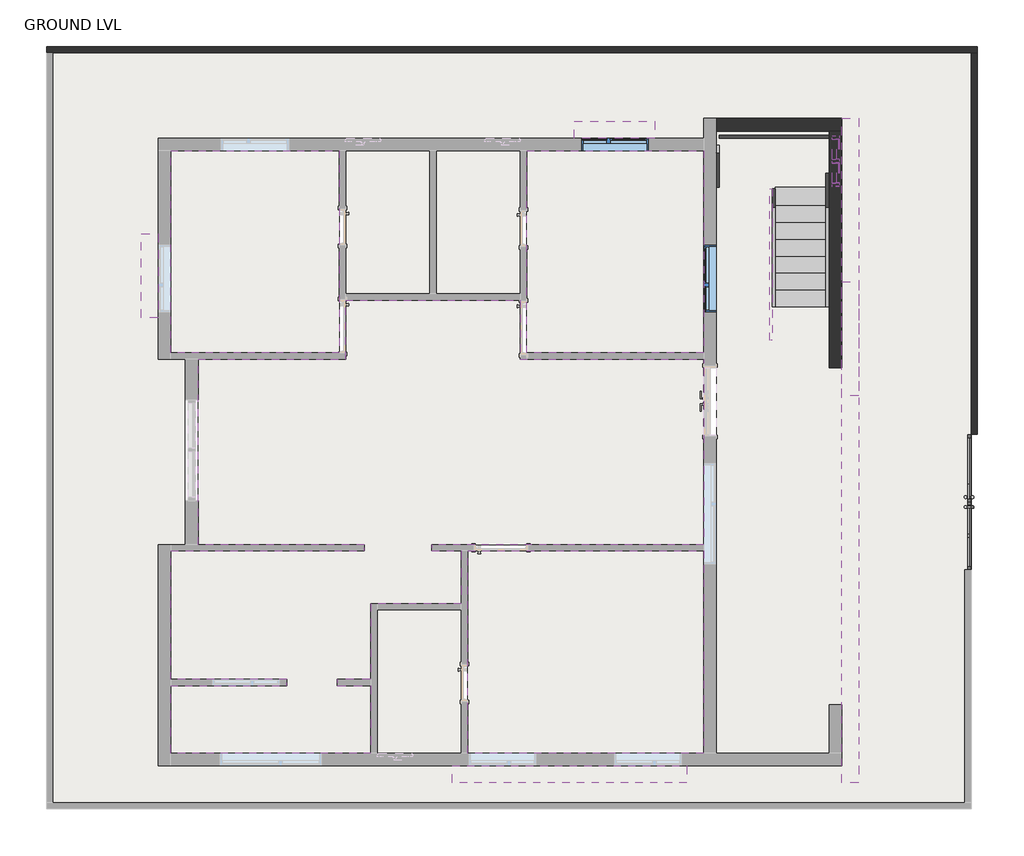
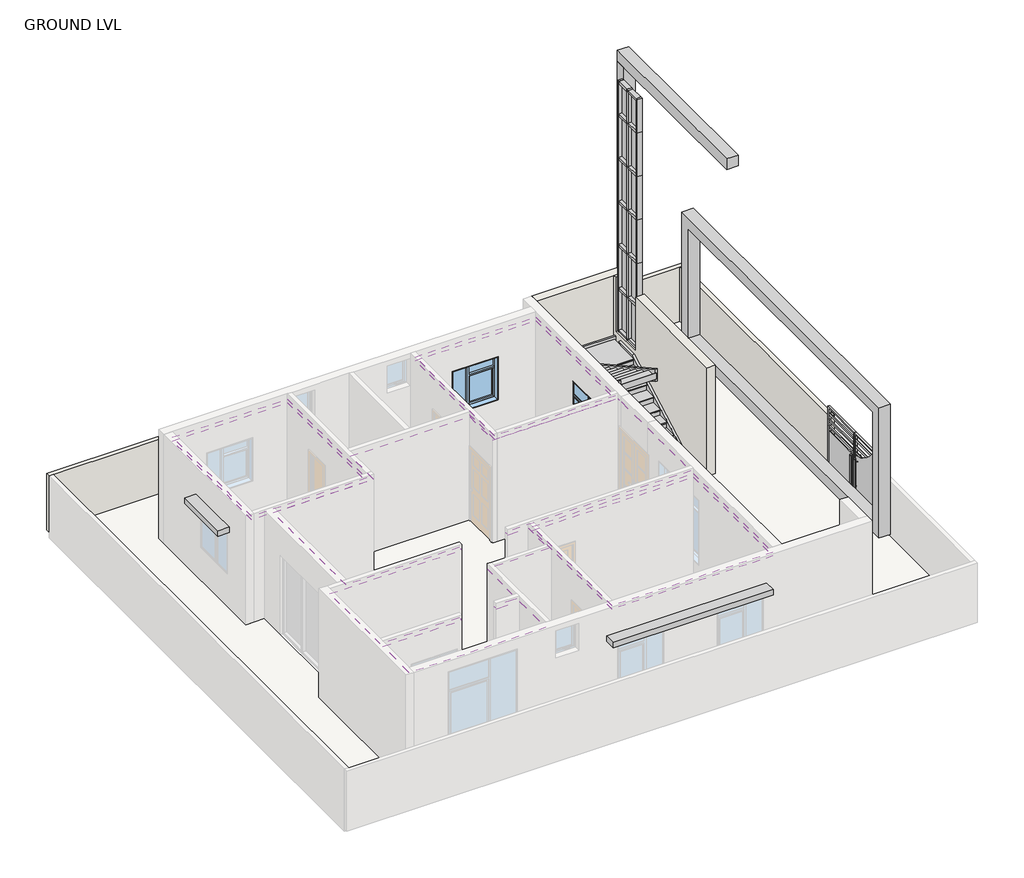
# One storey, part 2 of 2: 37 members, 12 plates, 10 coverings, 6 proxies, 4 walls, 3 slabs, 2 windows, 1 stair flight.
"""IFC4 building model written with IfcOpenShell, lengths in millimetres."""

from ifc_helpers import new_model, si_unit, frame, origin, place, context, project, spatial, polyline, outline, extrude, faceted_brep, transform, mapped, element, save
from components import generic_models_113f6068, generic_models_1_generic_models_1_001e7bd1, generic_models_2_generic_models_2_29e6902f, generic_models_4_generic_models_4_4e8aec35, generic_models_6_generic_models_6_966f38bf, generic_models_8_generic_models_8_43166a7e, member_75074519, member_f902c3b7, member_843225dc, member_af2f84b9, member_2b49869a, member_f2949ae1, system_panel_glazed_db5a8f8c, system_panel_glazed_28d38409, system_panel_glazed_f45b48ac, stair_flight_1848b3f0, window_casement_double_sidelight_window_4_x_4_2a492e8f

model = new_model("IFC4")

# Units and contexts
model_context = context("Model", 3, world=origin())
ifc_project = project(units=[si_unit("LENGTHUNIT", "METRE", prefix="MILLI")], contexts=[model_context])

# Site, building, storey
site = spatial("IfcSite", under=ifc_project)
building = spatial("IfcBuilding", under=site)
storey = spatial("IfcBuildingStorey", under=building, Name="GROUND LVL", Elevation=0.0)

# Proxies
placement = place(None, origin())
generic_models_shape = generic_models_113f6068(model_context)
element("IfcBuildingElementProxy", 1, Name="Generic Models", at=placement, inside=storey, context=model_context, shape_type="MappedRepresentation", body=[
    mapped(generic_models_shape, transform((25.4425412, 149.7000875, 0.0), x_axis=(0.0, 1.0, 0.0), y_axis=(-1.0, 0.0, 0.0), z_axis=(0.0, 0.0, 1.0))),
])
generic_models_1_generic_models_1_shape = generic_models_1_generic_models_1_001e7bd1(model_context)
element("IfcBuildingElementProxy", 2, Name="Generic Models 1 : Generic Models 1", ObjectType="Generic Models 1 : Generic Models 1", at=placement, inside=storey, context=model_context, shape_type="MappedRepresentation", body=[
    mapped(generic_models_1_generic_models_1_shape, transform((0.0, 0.0, 0.0), x_axis=(1.0, 0.0, 0.0), y_axis=(0.0, 1.0, 0.0), z_axis=(0.0, 0.0, 1.0))),
])
generic_models_2_generic_models_2_shape = generic_models_2_generic_models_2_29e6902f(model_context)
element("IfcBuildingElementProxy", 3, Name="Generic Models 2 : Generic Models 2", ObjectType="Generic Models 2 : Generic Models 2", at=placement, inside=storey, context=model_context, shape_type="MappedRepresentation", body=[
    mapped(generic_models_2_generic_models_2_shape, transform((0.0, 0.0, 0.0), x_axis=(1.0, 0.0, 0.0), y_axis=(0.0, 1.0, 0.0), z_axis=(0.0, 0.0, 1.0))),
])
generic_models_4_generic_models_4_shape = generic_models_4_generic_models_4_4e8aec35(model_context)
element("IfcBuildingElementProxy", 4, Name="Generic Models 5 : Generic Models 4", ObjectType="Generic Models 5 : Generic Models 4", at=placement, inside=storey, context=model_context, shape_type="MappedRepresentation", body=[
    mapped(generic_models_4_generic_models_4_shape, transform((0.0, 0.0, -3050.5796875), x_axis=(1.0, 0.0, 0.0), y_axis=(0.0, 1.0, 0.0), z_axis=(0.0, 0.0, 1.0))),
])
generic_models_6_generic_models_6_shape = generic_models_6_generic_models_6_966f38bf(model_context)
element("IfcBuildingElementProxy", 5, Name="Generic Models 6 : Generic Models 6", ObjectType="Generic Models 6 : Generic Models 6", at=placement, inside=storey, context=model_context, shape_type="MappedRepresentation", body=[
    mapped(generic_models_6_generic_models_6_shape, transform((0.0, 0.0, 0.0), x_axis=(1.0, 0.0, 0.0), y_axis=(0.0, 1.0, 0.0), z_axis=(0.0, 0.0, 1.0))),
])
generic_models_8_generic_models_8_shape = generic_models_8_generic_models_8_43166a7e(model_context)
element("IfcBuildingElementProxy", 6, Name="Generic Models 9 : Generic Models 8", ObjectType="Generic Models 9 : Generic Models 8", at=placement, inside=storey, context=model_context, shape_type="MappedRepresentation", body=[
    mapped(generic_models_8_generic_models_8_shape, transform((0.0, 0.0, -3048.0), x_axis=(1.0, 0.0, 0.0), y_axis=(0.0, 1.0, 0.0), z_axis=(0.0, 0.0, 1.0))),
])

# Coverings
element("IfcCovering", 7, ObjectType="GWB on Mtl. Stud", at=placement, inside=storey, context=model_context, shape_type="SweptSolid", body=[
    extrude(outline(polyline([(-12301.4656154, -3057.0499125), (-14396.9656154, -3057.0499125), (-14396.9656154, -732.9499125), (-10895.4913348, -732.9499125), (-10895.4913348, -618.6499125), (-13901.6656154, -618.6499125), (-13901.6656154, 2734.1500875), (-11234.6656154, 2734.1500875), (-11234.6656154, 3800.9500875), (-8072.3656154, 3800.9500875), (-8072.3656154, 2734.1500875), (-4757.6656154, 2734.1500875), (-4757.6656154, 2581.7500875), (-4757.6656154, 1362.5500875), (-4757.6656154, -618.6499125), (-9676.2913348, -618.6499125), (-9676.2913348, -732.9499125), (-9139.1656154, -732.9499125), (-9139.1656154, -1685.4499125), (-10777.4656154, -1685.4499125), (-10777.4656154, -3057.0499125), (-11387.0656154, -3057.0499125), (-11387.0656154, -3171.3499125), (-10777.4656154, -3171.3499125), (-10777.4656154, -4390.5499125), (-14396.9656154, -4390.5499125), (-14396.9656154, -3171.3499125), (-12301.4656154, -3171.3499125), (-12301.4656154, -3057.0499125)])), frame((0.0, 0.0, 2895.6), z_axis=(0.0, 0.0, 1.0), x_axis=(1.0, 0.0, 0.0)), (0.0, 0.0, 1.0), 107.95),
])
element("IfcCovering", 8, ObjectType="GWB on Mtl. Stud", at=placement, inside=storey, context=model_context, shape_type="SweptSolid", body=[
    extrude(outline(polyline([(-12301.4656154, -3057.0499125), (-14396.9656154, -3057.0499125), (-14396.9656154, -732.9499125), (-10895.4913348, -732.9499125), (-10895.4913348, -618.6499125), (-13901.6656154, -618.6499125), (-13901.6656154, 2734.1500875), (-11234.6656154, 2734.1500875), (-11234.6656154, 3800.9500875), (-8072.3656154, 3800.9500875), (-8072.3656154, 2734.1500875), (-4757.6656154, 2734.1500875), (-4757.6656154, 2581.7500875), (-4757.6656154, 1362.5500875), (-4757.6656154, -618.6499125), (-9676.2913348, -618.6499125), (-9676.2913348, -732.9499125), (-9139.1656154, -732.9499125), (-9139.1656154, -1685.4499125), (-10777.4656154, -1685.4499125), (-10777.4656154, -3057.0499125), (-11387.0656154, -3057.0499125), (-11387.0656154, -3171.3499125), (-10777.4656154, -3171.3499125), (-10777.4656154, -4390.5499125), (-14396.9656154, -4390.5499125), (-14396.9656154, -3171.3499125), (-12301.4656154, -3171.3499125), (-12301.4656154, -3057.0499125)])), frame((0.0, 0.0, 2895.6), z_axis=(0.0, 0.0, 1.0), x_axis=(1.0, 0.0, 0.0)), (0.0, 0.0, 1.0), 107.95),
])
element("IfcCovering", 9, ObjectType="GWB on Mtl. Stud", at=placement, inside=storey, context=model_context, shape_type="SweptSolid", body=[
    extrude(outline(polyline([(-12301.4656154, -3057.0499125), (-14396.9656154, -3057.0499125), (-14396.9656154, -732.9499125), (-10895.4913348, -732.9499125), (-10895.4913348, -618.6499125), (-13901.6656154, -618.6499125), (-13901.6656154, 2734.1500875), (-11234.6656154, 2734.1500875), (-11234.6656154, 3800.9500875), (-8072.3656154, 3800.9500875), (-8072.3656154, 2734.1500875), (-4757.6656154, 2734.1500875), (-4757.6656154, 2581.7500875), (-4757.6656154, 1362.5500875), (-4757.6656154, -618.6499125), (-9676.2913348, -618.6499125), (-9676.2913348, -732.9499125), (-9139.1656154, -732.9499125), (-9139.1656154, -1685.4499125), (-10777.4656154, -1685.4499125), (-10777.4656154, -3057.0499125), (-11387.0656154, -3057.0499125), (-11387.0656154, -3171.3499125), (-10777.4656154, -3171.3499125), (-10777.4656154, -4390.5499125), (-14396.9656154, -4390.5499125), (-14396.9656154, -3171.3499125), (-12301.4656154, -3171.3499125), (-12301.4656154, -3057.0499125)])), frame((0.0, 0.0, 2895.6), z_axis=(0.0, 0.0, 1.0), x_axis=(1.0, 0.0, 0.0)), (0.0, 0.0, 1.0), 107.95),
])
element("IfcCovering", 10, ObjectType="recessed ceiling", at=placement, inside=storey, context=model_context, shape_type="SweptSolid", body=[
    extrude(outline(polyline([(-14396.9656154, 2848.4500875), (-14396.9656154, 6506.0500875), (-11348.9656154, 6506.0500875), (-11348.9656154, 2848.4500875), (-14396.9656154, 2848.4500875)])), frame((0.0, 0.0, 2895.6), z_axis=(0.0, 0.0, 1.0), x_axis=(1.0, 0.0, 0.0)), (0.0, 0.0, 1.0), 107.95),
])
element("IfcCovering", 11, ObjectType="recessed ceiling", at=placement, inside=storey, context=model_context, shape_type="SweptSolid", body=[
    extrude(outline(polyline([(-11348.9656154, 6506.0500875), (-11348.9656154, 2848.4500875), (-14396.9656154, 2848.4500875), (-14396.9656154, 6506.0500875), (-11348.9656154, 6506.0500875)]), holes=[polyline([(-11653.7656154, 6201.2500875), (-14092.1656154, 6201.2500875), (-14092.1656154, 3153.2500875), (-11653.7656154, 3153.2500875), (-11653.7656154, 6201.2500875)])]), frame((0.0, 0.0, 2794.0), z_axis=(0.0, 0.0, 1.0), x_axis=(1.0, 0.0, 0.0)), (0.0, 0.0, 1.0), 107.95),
])
element("IfcCovering", 12, ObjectType="recessed ceiling", at=placement, inside=storey, context=model_context, shape_type="SweptSolid", body=[
    extrude(outline(polyline([(-7958.0656154, 2848.4500875), (-7958.0656154, 6506.0500875), (-4757.6656154, 6506.0500875), (-4757.6656154, 2848.4500875), (-7958.0656154, 2848.4500875)])), frame((0.0, 0.0, 2895.6), z_axis=(0.0, 0.0, 1.0), x_axis=(1.0, 0.0, 0.0)), (0.0, 0.0, 1.0), 107.95),
])
element("IfcCovering", 13, ObjectType="recessed ceiling", at=placement, inside=storey, context=model_context, shape_type="SweptSolid", body=[
    extrude(outline(polyline([(-4757.6656154, 6506.0500875), (-4757.6656154, 2848.4500875), (-7958.0656154, 2848.4500875), (-7958.0656154, 6506.0500875), (-4757.6656154, 6506.0500875)]), holes=[polyline([(-5062.4656154, 6201.2500875), (-7653.2656154, 6201.2500875), (-7653.2656154, 3153.2500875), (-5062.4656154, 3153.2500875), (-5062.4656154, 6201.2500875)])]), frame((0.0, 0.0, 2794.0), z_axis=(0.0, 0.0, 1.0), x_axis=(1.0, 0.0, 0.0)), (0.0, 0.0, 1.0), 107.95),
])
element("IfcCovering", 14, ObjectType="recessed ceiling", at=placement, inside=storey, context=model_context, shape_type="SweptSolid", body=[
    extrude(outline(polyline([(-4757.6656154, -732.9499125), (-4757.6656154, -4390.5499125), (-9024.8656154, -4390.5499125), (-9024.8656154, -732.9499125), (-4757.6656154, -732.9499125)])), frame((0.0, 0.0, 2895.6), z_axis=(0.0, 0.0, 1.0), x_axis=(1.0, 0.0, 0.0)), (0.0, 0.0, 1.0), 107.95),
])
element("IfcCovering", 15, ObjectType="recessed ceiling", at=placement, inside=storey, context=model_context, shape_type="SweptSolid", body=[
    extrude(outline(polyline([(-4757.6656154, -732.9499125), (-4757.6656154, -4390.5499125), (-9024.8656154, -4390.5499125), (-9024.8656154, -732.9499125), (-4757.6656154, -732.9499125)])), frame((0.0, 0.0, 2895.6), z_axis=(0.0, 0.0, 1.0), x_axis=(1.0, 0.0, 0.0)), (0.0, 0.0, 1.0), 107.95),
])
element("IfcCovering", 16, ObjectType="recessed ceiling", at=placement, inside=storey, context=model_context, shape_type="SweptSolid", body=[
    extrude(outline(polyline([(-4757.6656154, -732.9499125), (-4757.6656154, -4390.5499125), (-9024.8656154, -4390.5499125), (-9024.8656154, -732.9499125), (-4757.6656154, -732.9499125)]), holes=[polyline([(-5062.4656154, -1037.7499125), (-8720.0656154, -1037.7499125), (-8720.0656154, -4085.7499125), (-5062.4656154, -4085.7499125), (-5062.4656154, -1037.7499125)])]), frame((0.0, 0.0, 2794.0), z_axis=(0.0, 0.0, 1.0), x_axis=(1.0, 0.0, 0.0)), (0.0, 0.0, 1.0), 107.95),
])

# Members
member_shape = member_75074519(model_context)
element("IfcMember", 17, ObjectType="Rectangular Mullion : 2.5\" x 5\" rectangular", at=placement, inside=storey, context=model_context, shape_type="MappedRepresentation", body=[
    mapped(member_shape, transform((-2370.0656154, 5858.3500875, 3966.0038725), x_axis=(0.0, -1.0, 0.0), y_axis=(-1.0, 0.0, 0.0), z_axis=(0.0, 0.0, -1.0))),
])
element("IfcMember", 18, ObjectType="Rectangular Mullion : 2.5\" x 5\" rectangular", at=placement, inside=storey, context=model_context, shape_type="MappedRepresentation", body=[
    mapped(member_shape, transform((-2370.0656154, 5858.3500875, 6404.4038725), x_axis=(0.0, -1.0, 0.0), y_axis=(-1.0, 0.0, 0.0), z_axis=(0.0, 0.0, -1.0))),
])
element("IfcMember", 19, ObjectType="Rectangular Mullion : 2.5\" x 5\" rectangular", at=placement, inside=storey, context=model_context, shape_type="MappedRepresentation", body=[
    mapped(member_shape, transform((-2370.0656154, 5858.3500875, 5185.2038725), x_axis=(0.0, -1.0, 0.0), y_axis=(-1.0, 0.0, 0.0), z_axis=(0.0, 0.0, -1.0))),
])
element("IfcMember", 20, ObjectType="Rectangular Mullion : 2.5\" x 5\" rectangular", at=placement, inside=storey, context=model_context, shape_type="MappedRepresentation", body=[
    mapped(member_shape, transform((-2370.0656154, 5858.3500875, 2746.8038725), x_axis=(0.0, -1.0, 0.0), y_axis=(-1.0, 0.0, 0.0), z_axis=(0.0, 0.0, -1.0))),
])
element("IfcMember", 21, ObjectType="Rectangular Mullion : 2.5\" x 5\" rectangular", at=placement, inside=storey, context=model_context, shape_type="MappedRepresentation", body=[
    mapped(member_shape, transform((-2370.0656154, 6772.7500875, 3966.0038725), x_axis=(0.0, 1.0, 0.0), y_axis=(-1.0, 0.0, 0.0), z_axis=(0.0, 0.0, 1.0))),
])
element("IfcMember", 22, ObjectType="Rectangular Mullion : 2.5\" x 5\" rectangular", at=placement, inside=storey, context=model_context, shape_type="MappedRepresentation", body=[
    mapped(member_shape, transform((-2370.0656154, 6772.7500875, 6404.4038725), x_axis=(0.0, 1.0, 0.0), y_axis=(-1.0, 0.0, 0.0), z_axis=(0.0, 0.0, 1.0))),
])
element("IfcMember", 23, ObjectType="Rectangular Mullion : 2.5\" x 5\" rectangular", at=placement, inside=storey, context=model_context, shape_type="MappedRepresentation", body=[
    mapped(member_shape, transform((-2370.0656154, 6772.7500875, 7623.6038725), x_axis=(0.0, 1.0, 0.0), y_axis=(-1.0, 0.0, 0.0), z_axis=(0.0, 0.0, 1.0))),
])
element("IfcMember", 24, ObjectType="Rectangular Mullion : 2.5\" x 5\" rectangular", at=placement, inside=storey, context=model_context, shape_type="MappedRepresentation", body=[
    mapped(member_shape, transform((-2370.0656154, 6772.7500875, 5185.2038725), x_axis=(0.0, 1.0, 0.0), y_axis=(-1.0, 0.0, 0.0), z_axis=(0.0, 0.0, 1.0))),
])
element("IfcMember", 25, ObjectType="Rectangular Mullion : 2.5\" x 5\" rectangular", at=placement, inside=storey, context=model_context, shape_type="MappedRepresentation", body=[
    mapped(member_shape, transform((-2370.0656154, 5858.3500875, 1527.6038725), x_axis=(0.0, -1.0, 0.0), y_axis=(-1.0, 0.0, 0.0), z_axis=(0.0, 0.0, -1.0))),
])
element("IfcMember", 26, ObjectType="Rectangular Mullion : 2.5\" x 5\" rectangular", at=placement, inside=storey, context=model_context, shape_type="MappedRepresentation", body=[
    mapped(member_shape, transform((-2370.0656154, 6772.7500875, 2746.8038725), x_axis=(0.0, 1.0, 0.0), y_axis=(-1.0, 0.0, 0.0), z_axis=(0.0, 0.0, 1.0))),
])
member_2_shape = member_f902c3b7(model_context)
element("IfcMember", 27, ObjectType="Rectangular Mullion : 2.5\" x 5\" rectangular", at=placement, inside=storey, context=model_context, shape_type="MappedRepresentation", body=[
    mapped(member_2_shape, transform((-2370.0656154, 6772.7500875, 8564.5201514), x_axis=(0.0, 1.0, 0.0), y_axis=(-1.0, 0.0, 0.0), z_axis=(0.0, 0.0, 1.0))),
])
element("IfcMember", 28, ObjectType="Rectangular Mullion : 2.5\" x 5\" rectangular", at=placement, inside=storey, context=model_context, shape_type="MappedRepresentation", body=[
    mapped(member_2_shape, transform((-2370.0656154, 5858.3500875, 7623.6038725), x_axis=(0.0, -1.0, 0.0), y_axis=(-1.0, 0.0, 0.0), z_axis=(0.0, 0.0, -1.0))),
])
member_3_shape = member_843225dc(model_context)
element("IfcMember", 29, ObjectType="Rectangular Mullion : 2.5\" x 5\" rectangular", at=placement, inside=storey, context=model_context, shape_type="MappedRepresentation", body=[
    mapped(member_3_shape, transform((-2370.0656154, 5921.8500875, 8564.5201514), x_axis=(0.0, 0.0, 1.0), y_axis=(-1.0, 0.0, 0.0), z_axis=(0.0, -1.0, 0.0))),
])
element("IfcMember", 30, ObjectType="Rectangular Mullion : 2.5\" x 5\" rectangular", at=placement, inside=storey, context=model_context, shape_type="MappedRepresentation", body=[
    mapped(member_3_shape, transform((-2370.0656154, 6347.3000875, 8564.5201514), x_axis=(0.0, 0.0, 1.0), y_axis=(-1.0, 0.0, 0.0), z_axis=(0.0, -1.0, 0.0))),
])
element("IfcMember", 31, ObjectType="Rectangular Mullion : 2.5\" x 5\" rectangular", at=placement, inside=storey, context=model_context, shape_type="MappedRepresentation", body=[
    mapped(member_3_shape, transform((-2370.0656154, 6709.2500875, 1527.6038725), x_axis=(0.0, 0.0, -1.0), y_axis=(-1.0, 0.0, 0.0), z_axis=(0.0, 1.0, 0.0))),
])
element("IfcMember", 32, ObjectType="Rectangular Mullion : 2.5\" x 5\" rectangular", at=placement, inside=storey, context=model_context, shape_type="MappedRepresentation", body=[
    mapped(member_3_shape, transform((-2370.0656154, 6283.8000875, 1527.6038725), x_axis=(0.0, 0.0, -1.0), y_axis=(-1.0, 0.0, 0.0), z_axis=(0.0, 1.0, 0.0))),
])
member_4_shape = member_af2f84b9(model_context)
element("IfcMember", 33, ObjectType="Rectangular Mullion : 2.5\" x 5\" rectangular", at=placement, inside=storey, context=model_context, shape_type="MappedRepresentation", body=[
    mapped(member_4_shape, transform((-2370.0656154, 6347.3000875, 3966.0038725), x_axis=(0.0, 0.0, 1.0), y_axis=(-1.0, 0.0, 0.0), z_axis=(0.0, -1.0, 0.0))),
])
element("IfcMember", 34, ObjectType="Rectangular Mullion : 2.5\" x 5\" rectangular", at=placement, inside=storey, context=model_context, shape_type="MappedRepresentation", body=[
    mapped(member_4_shape, transform((-2370.0656154, 6347.3000875, 6404.4038725), x_axis=(0.0, 0.0, 1.0), y_axis=(-1.0, 0.0, 0.0), z_axis=(0.0, -1.0, 0.0))),
])
element("IfcMember", 35, ObjectType="Rectangular Mullion : 2.5\" x 5\" rectangular", at=placement, inside=storey, context=model_context, shape_type="MappedRepresentation", body=[
    mapped(member_4_shape, transform((-2370.0656154, 6347.3000875, 7623.6038725), x_axis=(0.0, 0.0, 1.0), y_axis=(-1.0, 0.0, 0.0), z_axis=(0.0, -1.0, 0.0))),
])
element("IfcMember", 36, ObjectType="Rectangular Mullion : 2.5\" x 5\" rectangular", at=placement, inside=storey, context=model_context, shape_type="MappedRepresentation", body=[
    mapped(member_4_shape, transform((-2370.0656154, 6347.3000875, 5185.2038725), x_axis=(0.0, 0.0, 1.0), y_axis=(-1.0, 0.0, 0.0), z_axis=(0.0, -1.0, 0.0))),
])
element("IfcMember", 37, ObjectType="Rectangular Mullion : 2.5\" x 5\" rectangular", at=placement, inside=storey, context=model_context, shape_type="MappedRepresentation", body=[
    mapped(member_4_shape, transform((-2370.0656154, 6347.3000875, 2746.8038725), x_axis=(0.0, 0.0, 1.0), y_axis=(-1.0, 0.0, 0.0), z_axis=(0.0, -1.0, 0.0))),
])
element("IfcMember", 38, ObjectType="Rectangular Mullion : 2.5\" x 5\" rectangular", at=placement, inside=storey, context=model_context, shape_type="MappedRepresentation", body=[
    mapped(member_4_shape, transform((-2370.0656154, 5921.8500875, 2746.8038725), x_axis=(0.0, 0.0, 1.0), y_axis=(-1.0, 0.0, 0.0), z_axis=(0.0, -1.0, 0.0))),
])
element("IfcMember", 39, ObjectType="Rectangular Mullion : 2.5\" x 5\" rectangular", at=placement, inside=storey, context=model_context, shape_type="MappedRepresentation", body=[
    mapped(member_4_shape, transform((-2370.0656154, 5921.8500875, 3966.0038725), x_axis=(0.0, 0.0, 1.0), y_axis=(-1.0, 0.0, 0.0), z_axis=(0.0, -1.0, 0.0))),
])
element("IfcMember", 40, ObjectType="Rectangular Mullion : 2.5\" x 5\" rectangular", at=placement, inside=storey, context=model_context, shape_type="MappedRepresentation", body=[
    mapped(member_4_shape, transform((-2370.0656154, 5921.8500875, 5185.2038725), x_axis=(0.0, 0.0, 1.0), y_axis=(-1.0, 0.0, 0.0), z_axis=(0.0, -1.0, 0.0))),
])
element("IfcMember", 41, ObjectType="Rectangular Mullion : 2.5\" x 5\" rectangular", at=placement, inside=storey, context=model_context, shape_type="MappedRepresentation", body=[
    mapped(member_4_shape, transform((-2370.0656154, 5921.8500875, 6404.4038725), x_axis=(0.0, 0.0, 1.0), y_axis=(-1.0, 0.0, 0.0), z_axis=(0.0, -1.0, 0.0))),
])
element("IfcMember", 42, ObjectType="Rectangular Mullion : 2.5\" x 5\" rectangular", at=placement, inside=storey, context=model_context, shape_type="MappedRepresentation", body=[
    mapped(member_4_shape, transform((-2370.0656154, 5921.8500875, 7623.6038725), x_axis=(0.0, 0.0, 1.0), y_axis=(-1.0, 0.0, 0.0), z_axis=(0.0, -1.0, 0.0))),
])
member_5_shape = member_2b49869a(model_context)
element("IfcMember", 43, ObjectType="Rectangular Mullion : 2.5\" x 5\" rectangular", at=placement, inside=storey, context=model_context, shape_type="MappedRepresentation", body=[
    mapped(member_5_shape, transform((-2370.0656154, 6315.5500875, 1527.6038725), x_axis=(0.0, -1.0, 0.0), y_axis=(-1.0, 0.0, 0.0), z_axis=(0.0, 0.0, -1.0))),
])
element("IfcMember", 44, ObjectType="Rectangular Mullion : 2.5\" x 5\" rectangular", at=placement, inside=storey, context=model_context, shape_type="MappedRepresentation", body=[
    mapped(member_5_shape, transform((-2370.0656154, 6315.5500875, 2746.8038725), x_axis=(0.0, -1.0, 0.0), y_axis=(-1.0, 0.0, 0.0), z_axis=(0.0, 0.0, -1.0))),
])
element("IfcMember", 45, ObjectType="Rectangular Mullion : 2.5\" x 5\" rectangular", at=placement, inside=storey, context=model_context, shape_type="MappedRepresentation", body=[
    mapped(member_5_shape, transform((-2370.0656154, 6315.5500875, 3966.0038725), x_axis=(0.0, -1.0, 0.0), y_axis=(-1.0, 0.0, 0.0), z_axis=(0.0, 0.0, -1.0))),
])
element("IfcMember", 46, ObjectType="Rectangular Mullion : 2.5\" x 5\" rectangular", at=placement, inside=storey, context=model_context, shape_type="MappedRepresentation", body=[
    mapped(member_5_shape, transform((-2370.0656154, 6315.5500875, 5185.2038725), x_axis=(0.0, -1.0, 0.0), y_axis=(-1.0, 0.0, 0.0), z_axis=(0.0, 0.0, -1.0))),
])
element("IfcMember", 47, ObjectType="Rectangular Mullion : 2.5\" x 5\" rectangular", at=placement, inside=storey, context=model_context, shape_type="MappedRepresentation", body=[
    mapped(member_5_shape, transform((-2370.0656154, 6315.5500875, 6404.4038725), x_axis=(0.0, -1.0, 0.0), y_axis=(-1.0, 0.0, 0.0), z_axis=(0.0, 0.0, -1.0))),
])
member_6_shape = member_f2949ae1(model_context)
element("IfcMember", 48, ObjectType="Rectangular Mullion : 2.5\" x 5\" rectangular", at=placement, inside=storey, context=model_context, shape_type="MappedRepresentation", body=[
    mapped(member_6_shape, transform((-2370.0656154, 6315.5500875, 7623.6038725), x_axis=(0.0, -1.0, 0.0), y_axis=(-1.0, 0.0, 0.0), z_axis=(0.0, 0.0, -1.0))),
])
element("IfcMember", 49, ObjectType="Stringer - 2\" Width", at=placement, inside=storey, context=model_context, shape_type="SweptSolid", body=[
    extrude(outline(polyline([(3686.6500875, 0.0), (3686.6500875, 207.5983948), (5751.3729769, 1354.6666667), (5820.2500875, 1354.6666667), (5820.2500875, 1044.253054), (3940.5945903, 0.0), (3686.6500875, 0.0)])), frame((-3513.0656154, 0.0, 0.0), z_axis=(1.0, 0.0, 0.0), x_axis=(0.0, 1.0, 0.0)), (0.0, 0.0, 1.0), 50.8),
])
element("IfcMember", 50, ObjectType="Stringer - 2\" Width", at=placement, inside=storey, context=model_context, shape_type="SweptSolid", body=[
    extrude(outline(polyline([(5820.2500875, 1562.2650614), (5820.2500875, 1213.5863873), (3077.0500875, 2737.5863873), (3077.0500875, 3086.2650614), (5820.2500875, 1562.2650614)])), frame((-3563.8656154, 0.0, 0.0), z_axis=(1.0, 0.0, 0.0), x_axis=(0.0, 1.0, 0.0)), (0.0, 0.0, 1.0), 50.8),
])
element("IfcMember", 51, ObjectType="Stringer - 2\" Width", at=placement, inside=storey, context=model_context, shape_type="SweptSolid", body=[
    extrude(outline(polyline([(3686.6500875, 0.0), (3686.6500875, 207.5983948), (5888.5329769, 1430.8666667), (6516.1545903, 1430.8666667), (3940.5945903, 0.0), (3686.6500875, 0.0)])), frame((-2547.8656154, 0.0, 0.0), z_axis=(1.0, 0.0, 0.0), x_axis=(0.0, 1.0, 0.0)), (0.0, 0.0, 1.0), 50.8),
])
element("IfcMember", 52, ObjectType="Stringer - 2\" Width", at=placement, inside=storey, context=model_context, shape_type="SweptSolid", body=[
    extrude(outline(polyline([(-2497.0656154, 6785.4500875), (-2497.0656154, 6734.6500875), (-4478.2656154, 6734.6500875), (-4478.2656154, 6785.4500875), (-2497.0656154, 6785.4500875)])), frame((0.0, 0.0, 1126.0666667), z_axis=(0.0, 0.0, 1.0), x_axis=(1.0, 0.0, 0.0)), (0.0, 0.0, 1.0), 304.8),
])
element("IfcMember", 53, ObjectType="Stringer - 2\" Width", at=placement, inside=storey, context=model_context, shape_type="SweptSolid", body=[
    extrude(outline(polyline([(5977.7855847, 1126.0666667), (3077.0500875, 2737.5863873), (3077.0500875, 3086.2650614), (6605.4071981, 1126.0666667), (5977.7855847, 1126.0666667)])), frame((-4529.0656154, 0.0, 0.0), z_axis=(1.0, 0.0, 0.0), x_axis=(0.0, 1.0, 0.0)), (0.0, 0.0, 1.0), 50.8),
])

# Plates
system_panel_glazed_shape = system_panel_glazed_db5a8f8c(model_context)
element("IfcPlate", 54, ObjectType="System Panel : Glazed", at=placement, inside=storey, context=model_context, shape_type="MappedRepresentation", body=[
    mapped(system_panel_glazed_shape, transform((-2370.0656154, 6528.2750875, 1591.1038725), x_axis=(0.0, -1.0, 0.0), y_axis=(1.0, 0.0, 0.0), z_axis=(0.0, 0.0, 1.0))),
])
element("IfcPlate", 55, ObjectType="System Panel : Glazed", at=placement, inside=storey, context=model_context, shape_type="MappedRepresentation", body=[
    mapped(system_panel_glazed_shape, transform((-2370.0656154, 6102.8250875, 1591.1038725), x_axis=(0.0, -1.0, 0.0), y_axis=(1.0, 0.0, 0.0), z_axis=(0.0, 0.0, 1.0))),
])
system_panel_glazed_2_shape = system_panel_glazed_28d38409(model_context)
element("IfcPlate", 56, ObjectType="System Panel : Glazed", at=placement, inside=storey, context=model_context, shape_type="MappedRepresentation", body=[
    mapped(system_panel_glazed_2_shape, transform((-2370.0656154, 6528.2750875, 3997.7538725), x_axis=(0.0, -1.0, 0.0), y_axis=(1.0, 0.0, 0.0), z_axis=(0.0, 0.0, 1.0))),
])
element("IfcPlate", 57, ObjectType="System Panel : Glazed", at=placement, inside=storey, context=model_context, shape_type="MappedRepresentation", body=[
    mapped(system_panel_glazed_2_shape, transform((-2370.0656154, 6528.2750875, 6436.1538725), x_axis=(0.0, -1.0, 0.0), y_axis=(1.0, 0.0, 0.0), z_axis=(0.0, 0.0, 1.0))),
])
element("IfcPlate", 58, ObjectType="System Panel : Glazed", at=placement, inside=storey, context=model_context, shape_type="MappedRepresentation", body=[
    mapped(system_panel_glazed_2_shape, transform((-2370.0656154, 6528.2750875, 5216.9538725), x_axis=(0.0, -1.0, 0.0), y_axis=(1.0, 0.0, 0.0), z_axis=(0.0, 0.0, 1.0))),
])
element("IfcPlate", 59, ObjectType="System Panel : Glazed", at=placement, inside=storey, context=model_context, shape_type="MappedRepresentation", body=[
    mapped(system_panel_glazed_2_shape, transform((-2370.0656154, 6528.2750875, 2778.5538725), x_axis=(0.0, -1.0, 0.0), y_axis=(1.0, 0.0, 0.0), z_axis=(0.0, 0.0, 1.0))),
])
element("IfcPlate", 60, ObjectType="System Panel : Glazed", at=placement, inside=storey, context=model_context, shape_type="MappedRepresentation", body=[
    mapped(system_panel_glazed_2_shape, transform((-2370.0656154, 6102.8250875, 2778.5538725), x_axis=(0.0, -1.0, 0.0), y_axis=(1.0, 0.0, 0.0), z_axis=(0.0, 0.0, 1.0))),
])
element("IfcPlate", 61, ObjectType="System Panel : Glazed", at=placement, inside=storey, context=model_context, shape_type="MappedRepresentation", body=[
    mapped(system_panel_glazed_2_shape, transform((-2370.0656154, 6102.8250875, 3997.7538725), x_axis=(0.0, -1.0, 0.0), y_axis=(1.0, 0.0, 0.0), z_axis=(0.0, 0.0, 1.0))),
])
element("IfcPlate", 62, ObjectType="System Panel : Glazed", at=placement, inside=storey, context=model_context, shape_type="MappedRepresentation", body=[
    mapped(system_panel_glazed_2_shape, transform((-2370.0656154, 6102.8250875, 5216.9538725), x_axis=(0.0, -1.0, 0.0), y_axis=(1.0, 0.0, 0.0), z_axis=(0.0, 0.0, 1.0))),
])
element("IfcPlate", 63, ObjectType="System Panel : Glazed", at=placement, inside=storey, context=model_context, shape_type="MappedRepresentation", body=[
    mapped(system_panel_glazed_2_shape, transform((-2370.0656154, 6102.8250875, 6436.1538725), x_axis=(0.0, -1.0, 0.0), y_axis=(1.0, 0.0, 0.0), z_axis=(0.0, 0.0, 1.0))),
])
system_panel_glazed_3_shape = system_panel_glazed_f45b48ac(model_context)
element("IfcPlate", 64, ObjectType="System Panel : Glazed", at=placement, inside=storey, context=model_context, shape_type="MappedRepresentation", body=[
    mapped(system_panel_glazed_3_shape, transform((-2370.0656154, 6528.2750875, 7655.3538725), x_axis=(0.0, -1.0, 0.0), y_axis=(1.0, 0.0, 0.0), z_axis=(0.0, 0.0, 1.0))),
])
element("IfcPlate", 65, ObjectType="System Panel : Glazed", at=placement, inside=storey, context=model_context, shape_type="MappedRepresentation", body=[
    mapped(system_panel_glazed_3_shape, transform((-2370.0656154, 6102.8250875, 7655.3538725), x_axis=(0.0, -1.0, 0.0), y_axis=(1.0, 0.0, 0.0), z_axis=(0.0, 0.0, 1.0))),
])

# Slabs
element("IfcSlab", 66, at=placement, inside=storey, context=model_context, shape_type="SweptSolid", body=[
    extrude(outline(polyline([(-9710.6656154, 6506.0500875), (-9710.6656154, 3915.2500875), (-11234.6656154, 3915.2500875), (-11234.6656154, 6506.0500875), (-9710.6656154, 6506.0500875)])), frame((0.0, 0.0, -152.4), z_axis=(0.0, 0.0, 1.0), x_axis=(1.0, 0.0, 0.0)), (0.0, 0.0, 1.0), 152.4),
    extrude(outline(polyline([(-8072.3656154, 6506.0500875), (-8072.3656154, 3915.2500875), (-9596.3656154, 3915.2500875), (-9596.3656154, 6506.0500875), (-8072.3656154, 6506.0500875)])), frame((0.0, 0.0, -152.4), z_axis=(0.0, 0.0, 1.0), x_axis=(1.0, 0.0, 0.0)), (0.0, 0.0, 1.0), 152.4),
    extrude(outline(polyline([(-9139.1656154, -1799.7499125), (-9139.1656154, -4390.5499125), (-10663.1656154, -4390.5499125), (-10663.1656154, -1799.7499125), (-9139.1656154, -1799.7499125)])), frame((0.0, 0.0, -152.4), z_axis=(0.0, 0.0, 1.0), x_axis=(1.0, 0.0, 0.0)), (0.0, 0.0, 1.0), 152.4),
])
element("IfcSlab", 67, ObjectType="ROSE MARBLE FLOOR", at=placement, inside=storey, context=model_context, shape_type="SweptSolid", body=[
    extrude(outline(polyline([(-11348.9656154, 6506.0500875), (-11348.9656154, 2848.4500875), (-14396.9656154, 2848.4500875), (-14396.9656154, 6506.0500875), (-11348.9656154, 6506.0500875)])), frame((0.0, 0.0, -152.4), z_axis=(0.0, 0.0, 1.0), x_axis=(1.0, 0.0, 0.0)), (0.0, 0.0, 1.0), 152.4),
    extrude(outline(polyline([(-4757.6656154, 6506.0500875), (-4757.6656154, 2848.4500875), (-7958.0656154, 2848.4500875), (-7958.0656154, 6506.0500875), (-4757.6656154, 6506.0500875)])), frame((0.0, 0.0, -152.4), z_axis=(0.0, 0.0, 1.0), x_axis=(1.0, 0.0, 0.0)), (0.0, 0.0, 1.0), 152.4),
    extrude(outline(polyline([(-13901.6656154, -618.6499125), (-13901.6656154, 2734.1500875), (-11234.6656154, 2734.1500875), (-11234.6656154, 3800.9500875), (-8072.3656154, 3800.9500875), (-8072.3656154, 2734.1500875), (-4757.6656154, 2734.1500875), (-4757.6656154, -618.6499125), (-9676.2913348, -618.6499125), (-9676.2913348, -732.9499125), (-9139.1656154, -732.9499125), (-9139.1656154, -1685.4499125), (-10777.4656154, -1685.4499125), (-10777.4656154, -3057.0499125), (-11387.0656154, -3057.0499125), (-11387.0656154, -3171.3499125), (-10777.4656154, -3171.3499125), (-10777.4656154, -4390.5499125), (-14396.9656154, -4390.5499125), (-14396.9656154, -3171.3499125), (-12301.4656154, -3171.3499125), (-12301.4656154, -3057.0499125), (-14396.9656154, -3057.0499125), (-14396.9656154, -732.9499125), (-10895.4913348, -732.9499125), (-10895.4913348, -618.6499125), (-13901.6656154, -618.6499125)])), frame((0.0, 0.0, -152.4), z_axis=(0.0, 0.0, 1.0), x_axis=(1.0, 0.0, 0.0)), (0.0, 0.0, 1.0), 152.4),
    extrude(outline(polyline([(-4757.6656154, -4390.5499125), (-9024.8656154, -4390.5499125), (-9024.8656154, -732.9499125), (-4757.6656154, -732.9499125), (-4757.6656154, -4390.5499125)])), frame((0.0, 0.0, -152.4), z_axis=(0.0, 0.0, 1.0), x_axis=(1.0, 0.0, 0.0)), (0.0, 0.0, 1.0), 152.4),
])
element("IfcSlab", 68, ObjectType="veranda marble", at=placement, inside=storey, context=model_context, shape_type="SweptSolid", body=[
    extrude(outline(polyline([(82.5925412, -5287.2307263), (-16529.0074588, -5287.2307263), (-16529.0074588, 8276.3692737), (82.5925412, 8276.3692737), (82.5925412, -5287.2307263)]), holes=[polyline([(-14625.5656154, -4619.1499125), (-4529.0656154, -4619.1499125), (-4529.0656154, 2581.7500875), (-4529.0656154, 6734.6500875), (-14625.5656154, 6734.6500875), (-14625.5656154, 2734.1500875), (-14130.2656154, 2734.1500875), (-14130.2656154, -618.6499125), (-14625.5656154, -618.6499125), (-14625.5656154, -4619.1499125)])]), frame((0.0, 0.0, -152.4), z_axis=(0.0, 0.0, 1.0), x_axis=(1.0, 0.0, 0.0)), (0.0, 0.0, 1.0), 152.4),
])

# Stair flight
stair_flight_shape = stair_flight_1848b3f0(model_context)
element("IfcStairFlight", 69, ObjectType="2\" Tread 1\" Nosing 1/4\" Riser", at=placement, inside=storey, context=model_context, shape_type="MappedRepresentation", body=[
    mapped(stair_flight_shape, transform((0.0, 0.0, 0.0), x_axis=(1.0, 0.0, 0.0), y_axis=(0.0, 1.0, 0.0), z_axis=(0.0, 0.0, 1.0))),
])

# Walls
element("IfcWall", 70, at=placement, inside=storey, context=model_context, shape_type="Brep", body=[
    faceted_brep([(-4529.0656154, 6861.6500875, 0.0), (-2484.3656154, 6861.6500875, 0.0), (-2255.7656154, 6861.6500875, 0.0), (-2255.7656154, 6861.6500875, 3048.0), (-2484.3656154, 6861.6500875, 3048.0), (-4529.0656154, 6861.6500875, 3048.0), (-4529.0656154, 7090.2500875, 0.0), (-4529.0656154, 7090.2500875, 3048.0), (-2255.7656154, 7090.2500875, 3048.0), (-2255.7656154, 7090.2500875, 0.0)], [[[0, 1, 2, 3, 4, 5]], [[6, 7, 8, 9]], [[2, 1, 0, 6, 9]], [[5, 4, 3, 8, 7]], [[0, 5, 7, 6]], [[3, 2, 9, 8]]]),
])
element("IfcWall", 71, at=placement, inside=storey, context=model_context, shape_type="SweptSolid", body=[
    extrude(outline(polyline([(6861.6500875, 0.0), (2581.7500875, 0.0), (2581.7500875, 3048.0), (5858.3500875, 3048.0), (5858.3500875, 1527.6038725), (6772.7500875, 1527.6038725), (6772.7500875, 3048.0), (6861.6500875, 3048.0), (6861.6500875, 0.0)])), frame((-2484.3656154, 0.0, 0.0), z_axis=(1.0, 0.0, 0.0), x_axis=(0.0, 1.0, 0.0)), (0.0, 0.0, 1.0), 228.6),
])
element("IfcWall", 72, at=placement, inside=storey, context=model_context, shape_type="Brep", body=[
    faceted_brep([(-16643.3074588, 8276.3692737, -59.3518251), (196.8925412, 8276.3692737, -59.3518251), (196.8925412, 8276.3692737, 1524.0), (82.5925412, 8276.3692737, 1524.0), (-16529.0074588, 8276.3692737, 1524.0), (-16643.3074588, 8276.3692737, 1524.0), (-16643.3074588, 8390.6692737, -59.3518251), (-16643.3074588, 8390.6692737, 1524.0), (196.8925412, 8390.6692737, 1524.0), (196.8925412, 8390.6692737, -59.3518251)], [[[0, 1, 2, 3, 4, 5]], [[6, 7, 8, 9]], [[1, 0, 6, 9]], [[5, 4, 3, 2, 8, 7]], [[0, 5, 7, 6]], [[2, 1, 9, 8]]]),
])
element("IfcWall", 73, at=placement, inside=storey, context=model_context, shape_type="Brep", body=[
    faceted_brep([(82.5925412, 8276.3692737, -152.4), (82.5925412, 1373.9192737, -152.4), (82.5925412, 1373.9192737, 1524.0), (82.5925412, 8276.3692737, 1524.0), (196.8925412, 8276.3692737, -152.4), (196.8925412, 8276.3692737, -59.3518251), (196.8925412, 8276.3692737, 1524.0), (196.8925412, 1373.9192737, 1524.0), (196.8925412, 1373.9192737, -152.4)], [[[0, 1, 2, 3]], [[4, 5, 6, 7, 8]], [[1, 0, 4, 8]], [[2, 1, 8, 7]], [[3, 2, 7, 6]], [[0, 3, 6, 5, 4]]]),
])

# Windows
window_casement_double_sidelight_window_4_x_4_shape = window_casement_double_sidelight_window_4_x_4_2a492e8f(model_context)
element("IfcWindow", 74, ObjectType="Window-Casement-Double-Sidelight : window 4' x 4'", at=placement, inside=storey, context=model_context, shape_type="MappedRepresentation", body=[
    mapped(window_casement_double_sidelight_window_4_x_4_shape, transform((-6357.8656154, 6620.3500875, 0.0), x_axis=(1.0, 0.0, 0.0), y_axis=(0.0, 1.0, 0.0), z_axis=(0.0, 0.0, 1.0))),
])
element("IfcWindow", 75, ObjectType="Window-Casement-Double-Sidelight : window 4' x 4'", at=placement, inside=storey, context=model_context, shape_type="MappedRepresentation", body=[
    mapped(window_casement_double_sidelight_window_4_x_4_shape, transform((-4643.3656154, 4193.5295492, 0.0), x_axis=(0.0, 1.0, 0.0), y_axis=(-1.0, 0.0, 0.0), z_axis=(0.0, 0.0, 1.0))),
])

save(model, "model.ifc")

# Revit data of these elements
# Type
#   sheet = none
#   pipe = none
#   handal = none
#   faram = none
#   Default Elevation = 0
# Type "GWB on Mtl. Stud"
#   Assembly Code = "C3030220"
#   built-in parameter 1002203 = 1 (stored number, unit not read)
#   built-in parameter 1002202 = 1 (stored number, unit not read)
#   Layers, outside or top first: 0' - 3 5/8" "Metal Stud Layer" (function 1); 0' - 0 5/8" "Gypsum Wall Board" (function 5)
# Type "recessed ceiling"
#   Assembly Code = "C3030220"
#   built-in parameter 1002203 = 1 (stored number, unit not read)
#   built-in parameter 1002202 = 1 (stored number, unit not read)
#   Layers, outside or top first: 0' - 3 5/8" "recessed ceiling" (function 1); 0' - 0 5/8" "LIGHT BEIGE" (function 5)
# Type "Rectangular Mullion : 2.5\" x 5\" rectangular"
#   built-in parameter 1007304 = 0.416667 (stored number, unit not read)
#   built-in parameter 1007301 = 0.104167 (stored number, unit not read)
#   built-in parameter 1007300 = 0.104167 (stored number, unit not read)
# Type "System Panel : Glazed"
#   Construction Type Id = "GSP4R"
#   Analytic Construction = "1/8 in Pilkington single glazing"
#   Visual Light Transmittance = 0.9
#   Solar Heat Gain Coefficient = 0.86
#   Heat Transfer Coefficient (U) = 1.18115 BTU/(h·ft²·°F)
#   Define Thermal Properties by = 1
# Type
#   Assembly Code = "B1010"
#   Function = 0
# Type "ROSE MARBLE FLOOR"
#   Assembly Code = "B1010"
#   Function = 0
#   Layers, outside or top first: 0' - 6" "MARBLE FLOORING" (function 1)
# Type "veranda marble"
#   Assembly Code = "B1010"
#   Function = 0
#   Layers, outside or top first: 0' - 6" "outer flooring" (function 1)
# Type
#   Assembly Code = "B2010"
#   Layers, outside or top first: 0' - 9" "LIGHT BEIGE" (function 1)
# Type
#   Assembly Code = "B2010"
#   Layers, outside or top first: 0' - 4 1/2" "LIGHT BEIGE" (function 1)
# Type "Window-Casement-Double-Sidelight : window 4' x 4'"
#   Type Mark = "22"
#   Fire Rating = "0.5h"
#   Assembly Code = "B2020100"
#   Analytic Construction = "Double glazing - domestic"
#   Window Inset [instance default] = 0' - 0 5/8"
#   Wall Thickness [instance default] = 0' - 6"
#   Visual Light Transmittance = 0.81
#   Transom Height Ratio = 0.3
#   Transom Height = 1' - 2.4"
#   Thermal Resistance (R) = 1.8146 (h·ft²·°F)/BTU
#   Solar Heat Gain Coefficient = 0.76
#   Side Width = 1' - 7.2"
#   Rough Width = 4' - 0 1/2"
#   Rough Height = 4' - 0 1/2"
#   Opening Window Width = 2' - 4.8"
#   Opening Window Height = 2' - 9.6"
#   Heat Transfer Coefficient (U) = 0.5511 BTU/(h·ft²·°F)
#   Height = 4' - 0"
#   Frame Gap 3 [instance default] = 0' - 1 83/128"
#   Frame Gap 2 [instance default] = 0' - 0 5/8"
#   Frame Gap 1 = 0' - 1 51/128"
#   Default Sill Height = 3' - 0"
#   Width = 4' - 0"
#   Frame Material = Metal - Aluminum
#   Glass Panel Material = Glass
#   Wall Closure = (empty or 0)
# Element 1 (IfcBuildingElementProxy)
#   Phase Created = New Construction
#   Materials on its faces: "Earth"
# Element 2 (IfcBuildingElementProxy, "Generic Models 1 : Generic Models 1")
#   Phase Created = New Construction
#   Materials on its faces: "LIGHT BEIGE"
# Element 3 (IfcBuildingElementProxy, "Generic Models 2 : Generic Models 2")
#   Phase Created = New Construction
#   Materials on its faces: "LIGHT BEIGE"
# Element 4 (IfcBuildingElementProxy, "Generic Models 5 : Generic Models 4")
#   Phase Created = New Construction
#   Materials on its faces: "LIGHT BEIGE"
# Element 5 (IfcBuildingElementProxy, "Generic Models 6 : Generic Models 6")
#   Phase Created = New Construction
#   Materials on its faces: "LIGHT BEIGE"
# Element 6 (IfcBuildingElementProxy, "Generic Models 9 : Generic Models 8")
#   Phase Created = New Construction
#   Materials on its faces: "LIGHT BEIGE"
# Elements 7, 8, 9 (IfcCovering, "GWB on Mtl. Stud")
#   Height Offset From Level = 9' - 6"
#   Phase Created = New Construction
#   Materials on its faces: "Gypsum Wall Board", "Metal Stud Layer"
# Elements 10, 12, 14, 15 (IfcCovering, "recessed ceiling")
#   Height Offset From Level = 9' - 6"
#   Phase Created = New Construction
#   Materials on its faces: "LIGHT BEIGE", "recessed ceiling"
# Elements 11, 13, 16 (IfcCovering, "recessed ceiling")
#   Height Offset From Level = 9' - 2"
#   Phase Created = New Construction
#   Materials on its faces: "LIGHT BEIGE", "recessed ceiling"
# Elements 17, 18, 19, 20, 21, 22, 23, 24, 25, 26, 27, 28, 29, 30, 31, 32, 33, 34, 35, 36, 37, 38, 39, 40, 41, 42, 43, 44, 45, 46, 47, 48 (IfcMember, "Rectangular Mullion : 2.5\" x 5\" rectangular")
#   Phase Created = New Construction
#   Materials on its faces: "Aluminum"
# Elements 49, 50, 51, 52, 53 (IfcMember, "Stringer - 2\" Width")
#   Phase Created = New Construction
# Elements 54, 55, 56, 57, 58, 59, 60, 61, 62, 63, 64, 65 (IfcPlate, "System Panel : Glazed")
#   Phase Created = New Construction
#   Materials on its faces: "Glass"
# Element 66 (IfcSlab)
#   Height Offset From Level = 0' - 0"
#   Phase Created = New Construction
# Element 67 (IfcSlab, "ROSE MARBLE FLOOR")
#   Height Offset From Level = 0' - 0"
#   Phase Created = New Construction
#   Materials on its faces: "MARBLE FLOORING"
# Element 68 (IfcSlab, "veranda marble")
#   Height Offset From Level = 0' - 0"
#   Phase Created = New Construction
#   Materials on its faces: "outer flooring"
# Element 69 (IfcStairFlight, "2\" Tread 1\" Nosing 1/4\" Riser")
#   Phase Created = New Construction
# Elements 70, 71 (IfcWall)
#   Top Offset = 0' - 0"
#   Base Offset = 0' - 0"
#   wall height = 10' - 0"
#   Phase Created = New Construction
#   Base Constraint = GROUND LVL
#   Top Constraint = FIRST FLOOR
#   Materials on its faces: "LIGHT BEIGE"
# Element 72 (IfcWall)
#   built-in parameter 1001111 = -0' - 2.33669"
#   Top Offset = 0' - 0"
#   Base Offset = -0' - 2.33669"
#   Unconnected Height = 5' - 2.33669"
#   wall height = 5' - 2.33669"
#   Phase Created = New Construction
#   Base Constraint = GROUND LVL
#   Materials on its faces: "LIGHT BEIGE"
# Element 73 (IfcWall)
#   built-in parameter 1001111 = -0' - 6"
#   Top Offset = 0' - 0"
#   Base Offset = -0' - 6"
#   Unconnected Height = 5' - 6"
#   wall height = 5' - 6"
#   Phase Created = New Construction
#   Base Constraint = GROUND LVL
#   Materials on its faces: "LIGHT BEIGE"
# Element 74 (IfcWindow, "Window-Casement-Double-Sidelight : window 4' x 4'")
#   Mark = "10"
#   Window Inset = 0' - 0 5/8"
#   Frame Gap 3 = 0' - 1 83/128"
#   Frame Gap 2 = 0' - 0 5/8"
#   Phase Created = New Construction
#   Materials on its faces: "Metal - Aluminum", "Glass"
# Element 75 (IfcWindow, "Window-Casement-Double-Sidelight : window 4' x 4'")
#   Mark = "13"
#   Window Inset = 0' - 0 5/8"
#   Frame Gap 3 = 0' - 1 83/128"
#   Frame Gap 2 = 0' - 0 5/8"
#   Phase Created = New Construction
#   Materials on its faces: "Metal - Aluminum", "Glass"
# Materials
#   "Metal Stud Layer": class "Metal", colour RGB 199 199 199, transparency 0, Description = "Light gauge steel framing, thermal air layer", Cost = 0
#   "Gypsum Wall Board": class "Generic", colour RGB 127 127 127, transparency 0, Description = "Gypsum Wall Board", Cost = 0
#   "recessed ceiling": class "Generic", colour RGB 120 120 120, transparency 0, Cost = 0
#   "LIGHT BEIGE": class "Generic", colour RGB 120 120 120, transparency 0, Cost = 0
#   "MARBLE FLOORING": class "Generic", colour RGB 120 120 120, transparency 0, Cost = 0
#   "outer flooring": class "Generic", colour RGB 120 120 120, transparency 0, Cost = 0
#   "Metal - Aluminum": class "Metal", colour RGB 247 247 247, transparency 0
#   "Glass": class "Glass", colour RGB 0 128 192, transparency 0.75, Description = "Soda Lime Glass", Cost = 0
#   "Earth": class "Generic", colour RGB 97 75 62, transparency 0, Description = "Soil", Cost = 0
#   "Aluminum": class "Metal", colour RGB 247 247 247, transparency 0, Description = "Aluminum 6061", Cost = 0
